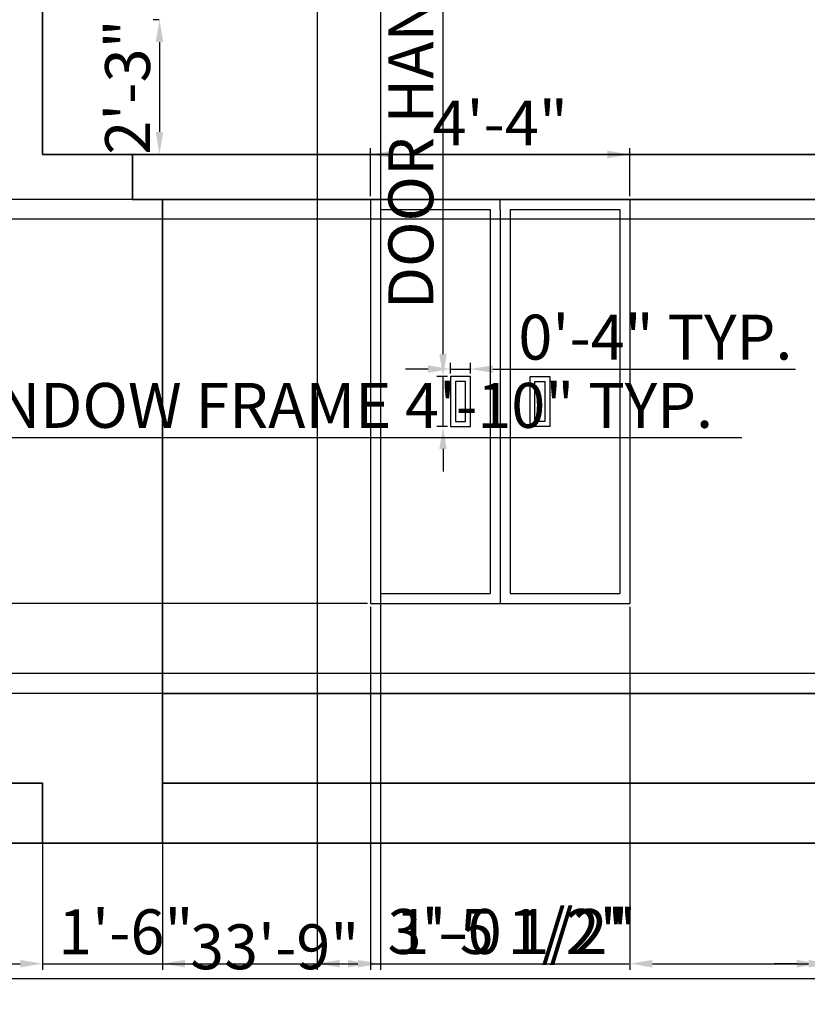
# Model space of a CAD drawing. Units: inches. Extents: x 3297 to 3846, y 520 to 959.
# Tile 2 of 5: x 3483 to 3641, y 520 to 717. Entities that reach past the tile are written whole.
import ezdxf

# ---------------------------------------------------------------- set-up
doc = ezdxf.new("R2010")
doc.units = ezdxf.units.IN
for name, color, linetype, lineweight in [('A-ANNO-DIMS', 2, 'Continuous', 18), ('A-DOOR', 4, 'Continuous', 25), ('A-ELEV', 7, 'Continuous', 35)]:
    doc.layers.add(name, color=color, linetype=linetype, lineweight=lineweight)
doc.styles.get("Standard").update_dxf_attribs({"font": 'arial.ttf'})
doc.dimstyles.new('ISO-25', dxfattribs={"dimtxt": 9, "dimasz": 4.5, "dimexe": 1.25, "dimexo": 0.625, "dimtad": 1, "dimdec": 0, "dimlunit": 3, "dimtxsty": 'Standard', "dimcen": 2.5, "dimadec": 0, "dimazin": 0, "dimtfac": 1, "dimtdec": 0, "dimtmove": 0, "dimatfit": 3, "dimfxl": 1, "dimarcsym": 0})

# ---------------------------------------------------------------- blocks, each defined once
blk = doc.blocks.new('*D7')
at = {"layer": 'A-ANNO-DIMS', "color": 0, "lineweight": -2, "transparency": 16777216}
for p, q in [((3332.06, 551.62), (3332.06, 523.84)), ((3737.06, 551.62), (3737.06, 523.84)), ((3336.56, 525.09), (3732.56, 525.09))]:
    blk.add_line(p, q, dxfattribs=at)
at = {"layer": 'A-ANNO-DIMS', "color": 0, "transparency": 16777216}
for points in [[(3336.56, 525.84), (3336.56, 524.34), (3332.06, 525.09)], [(3732.56, 525.84), (3732.56, 524.34), (3737.06, 525.09)]]:
    blk.add_solid(points, dxfattribs=at)
at = {"layer": 'Defpoints', "color": 0, "transparency": 16777216}
for p in [(3332.06, 552.24), (3737.06, 552.24), (3737.06, 525.09)]:
    blk.add_point(p, dxfattribs=at)
at = {"layer": 'A-ANNO-DIMS', "color": 0, "transparency": 16777216, "insert": (3534.56, 530.31), "char_height": 9, "attachment_point": 5}
blk.add_mtext('33\'-9"', dxfattribs=at)
blk = doc.blocks.new('*D12')
at = {"layer": 'A-ANNO-DIMS', "color": 0, "lineweight": -2, "transparency": 16777216}
for p, q in [((3553.76, 681.87), (3553.76, 691.49)), ((3605.76, 681.87), (3605.76, 691.49)), ((3558.26, 690.24), (3601.26, 690.24))]:
    blk.add_line(p, q, dxfattribs=at)
at = {"layer": 'A-ANNO-DIMS', "color": 0, "transparency": 16777216}
for points in [[(3558.26, 690.99), (3558.26, 689.49), (3553.76, 690.24)], [(3601.26, 690.99), (3601.26, 689.49), (3605.76, 690.24)]]:
    blk.add_solid(points, dxfattribs=at)
at = {"layer": 'Defpoints', "color": 0, "transparency": 16777216}
for p in [(3605.76, 690.24), (3553.76, 681.24), (3605.76, 681.24)]:
    blk.add_point(p, dxfattribs=at)
at = {"layer": 'A-ANNO-DIMS', "color": 0, "transparency": 16777216, "insert": (3579.76, 695.37), "char_height": 9, "attachment_point": 5}
blk.add_mtext('4\'-4"', dxfattribs=at)
blk = doc.blocks.new('*D19')
at = {"layer": 'A-ANNO-DIMS', "color": 0, "lineweight": -2, "transparency": 16777216}
for p, q in [((3511.44, 717.24), (3510.23, 717.24)), ((3511.48, 712.74), (3511.48, 694.74)), ((3511.44, 690.24), (3510.23, 690.24))]:
    blk.add_line(p, q, dxfattribs=at)
at = {"layer": 'A-ANNO-DIMS', "color": 0, "transparency": 16777216}
for points in [[(3510.73, 712.74), (3512.23, 712.74), (3511.48, 717.24)], [(3510.73, 694.74), (3512.23, 694.74), (3511.48, 690.24)]]:
    blk.add_solid(points, dxfattribs=at)
at = {"layer": 'Defpoints', "color": 0, "transparency": 16777216}
for p in [(3512.06, 717.24), (3511.48, 690.24), (3512.06, 690.24)]:
    blk.add_point(p, dxfattribs=at)
at = {"layer": 'A-ANNO-DIMS', "color": 0, "transparency": 16777216, "insert": (3506.25, 703.74), "char_height": 9, "attachment_point": 5, "rotation": 90}
blk.add_mtext('2\'-3"', dxfattribs=at)
blk = doc.blocks.new('DOOR-HANDLE')
for points in [[(3573.8, 645.74), (3569.8, 645.74), (3569.8, 640.74), (3569.8, 635.74), (3573.8, 635.74), (3573.8, 640.74)], [(3572.8, 644.74), (3570.8, 644.74), (3570.8, 640.74), (3570.8, 636.74), (3572.8, 636.74), (3572.8, 640.74)]]:
    blk.add_lwpolyline(points, close=True)
blk = doc.blocks.new('*D29')
at = {"layer": 'A-ANNO-DIMS', "color": 0, "lineweight": -2, "transparency": 16777216}
for p, q in [((3568.3, 650.24), (3568.3, 813.1)), ((3569.18, 645.74), (3567.05, 645.74)), ((3568.3, 635.74), (3568.3, 645.74)), ((3569.18, 635.74), (3567.05, 635.74)), ((3568.3, 631.24), (3568.3, 626.74))]:
    blk.add_line(p, q, dxfattribs=at)
at = {"layer": 'A-ANNO-DIMS', "color": 0, "transparency": 16777216}
for points in [[(3567.55, 650.24), (3569.05, 650.24), (3568.3, 645.74)], [(3567.55, 631.24), (3569.05, 631.24), (3568.3, 635.74)]]:
    blk.add_solid(points, dxfattribs=at)
at = {"layer": 'Defpoints', "color": 0, "transparency": 16777216}
for p in [(3568.3, 645.74), (3569.8, 645.74), (3569.8, 635.74)]:
    blk.add_point(p, dxfattribs=at)
at = {"layer": 'A-ANNO-DIMS', "color": 0, "transparency": 16777216, "insert": (3563.02, 733.92), "char_height": 9, "attachment_point": 5, "rotation": 90}
blk.add_mtext('DOOR HANDLE 0\'-10" TYP.', dxfattribs=at)
blk = doc.blocks.new('*D30')
at = {"layer": 'A-ANNO-DIMS', "color": 0, "lineweight": -2, "transparency": 16777216}
for p, q in [((3565.3, 647.24), (3560.8, 647.24)), ((3569.8, 646.37), (3569.8, 648.49)), ((3569.8, 647.24), (3573.8, 647.24)), ((3573.8, 646.37), (3573.8, 648.49)), ((3578.3, 647.24), (3638.91, 647.24))]:
    blk.add_line(p, q, dxfattribs=at)
at = {"layer": 'A-ANNO-DIMS', "color": 0, "transparency": 16777216}
for points in [[(3565.3, 647.99), (3565.3, 646.49), (3569.8, 647.24)], [(3578.3, 647.99), (3578.3, 646.49), (3573.8, 647.24)]]:
    blk.add_solid(points, dxfattribs=at)
at = {"layer": 'Defpoints', "color": 0, "transparency": 16777216}
for p in [(3573.8, 647.24), (3569.8, 645.74), (3573.8, 645.74)]:
    blk.add_point(p, dxfattribs=at)
at = {"layer": 'A-ANNO-DIMS', "color": 0, "transparency": 16777216, "insert": (3610.86, 652.46), "char_height": 9, "attachment_point": 5}
blk.add_mtext('0\'-4" TYP.', dxfattribs=at)
blk = doc.blocks.new('*D31')
at = {"layer": 'A-ANNO-DIMS', "color": 0, "lineweight": -2, "transparency": 16777216}
for p, q in [((3396.06, 641.58), (3396.06, 632.26)), ((3454.06, 641.58), (3454.06, 632.26)), ((3400.56, 633.51), (3449.56, 633.51)), ((3454.06, 633.51), (3628.19, 633.51))]:
    blk.add_line(p, q, dxfattribs=at)
at = {"layer": 'A-ANNO-DIMS', "color": 0, "transparency": 16777216}
for points in [[(3400.56, 634.26), (3400.56, 632.76), (3396.06, 633.51)], [(3449.56, 634.26), (3449.56, 632.76), (3454.06, 633.51)]]:
    blk.add_solid(points, dxfattribs=at)
at = {"layer": 'Defpoints', "color": 0, "transparency": 16777216}
for p in [(3396.06, 642.21), (3454.06, 642.21), (3454.06, 633.51)]:
    blk.add_point(p, dxfattribs=at)
at = {"layer": 'A-ANNO-DIMS', "color": 0, "transparency": 16777216, "insert": (3543.38, 638.79), "char_height": 9, "attachment_point": 5}
blk.add_mtext('WINDOW FRAME 4\'-10" TYP.', dxfattribs=at)
blk = doc.blocks.new('*D51')
at = {"layer": 'A-ANNO-DIMS', "color": 0, "lineweight": -2, "transparency": 16777216}
for p, q in [((3646.06, 575.62), (3646.06, 526.84)), ((3643.69, 563.62), (3643.69, 526.84)), ((3639.19, 528.09), (3634.69, 528.09)), ((3643.69, 528.09), (3646.06, 528.09)), ((3650.56, 528.09), (3701.21, 528.09))]:
    blk.add_line(p, q, dxfattribs=at)
at = {"layer": 'A-ANNO-DIMS', "color": 0, "transparency": 16777216}
for points in [[(3639.19, 528.84), (3639.19, 527.34), (3643.69, 528.09)], [(3650.56, 528.84), (3650.56, 527.34), (3646.06, 528.09)]]:
    blk.add_solid(points, dxfattribs=at)
at = {"layer": 'Defpoints', "color": 0, "transparency": 16777216}
for p in [(3646.06, 576.24), (3643.69, 564.24), (3646.06, 528.09)]:
    blk.add_point(p, dxfattribs=at)
at = {"layer": 'A-ANNO-DIMS', "color": 0, "transparency": 16777216, "insert": (3678.14, 533.37), "char_height": 9, "attachment_point": 5}
blk.add_mtext('0\'-2 1/2"', dxfattribs=at)
blk = doc.blocks.new('*D52')
at = {"layer": 'A-ANNO-DIMS', "color": 0, "lineweight": -2, "transparency": 16777216}
for p, q in [((3553.76, 599.62), (3553.76, 526.84)), ((3512.06, 581.62), (3512.06, 526.84)), ((3516.56, 528.09), (3549.26, 528.09)), ((3553.76, 528.09), (3604.4, 528.09))]:
    blk.add_line(p, q, dxfattribs=at)
at = {"layer": 'A-ANNO-DIMS', "color": 0, "transparency": 16777216}
for points in [[(3516.56, 528.84), (3516.56, 527.34), (3512.06, 528.09)], [(3549.26, 528.84), (3549.26, 527.34), (3553.76, 528.09)]]:
    blk.add_solid(points, dxfattribs=at)
at = {"layer": 'Defpoints', "color": 0, "transparency": 16777216}
for p in [(3553.76, 600.24), (3512.06, 582.24), (3553.76, 528.09)]:
    blk.add_point(p, dxfattribs=at)
at = {"layer": 'A-ANNO-DIMS', "color": 0, "transparency": 16777216, "insert": (3581.33, 533.37), "char_height": 9, "attachment_point": 5}
blk.add_mtext('3\'-5 1/2"', dxfattribs=at)
blk = doc.blocks.new('*D53')
at = {"layer": 'A-ANNO-DIMS', "color": 0, "lineweight": -2, "transparency": 16777216}
for p, q in [((3605.76, 599.62), (3605.76, 526.84)), ((3646.06, 581.62), (3646.06, 526.84)), ((3610.26, 528.09), (3641.56, 528.09)), ((3646.06, 528.09), (3696.7, 528.09))]:
    blk.add_line(p, q, dxfattribs=at)
at = {"layer": 'A-ANNO-DIMS', "color": 0, "transparency": 16777216}
for points in [[(3610.26, 528.84), (3610.26, 527.34), (3605.76, 528.09)], [(3641.56, 528.84), (3641.56, 527.34), (3646.06, 528.09)]]:
    blk.add_solid(points, dxfattribs=at)
at = {"layer": 'Defpoints', "color": 0, "transparency": 16777216}
for p in [(3605.76, 600.24), (3646.06, 582.24), (3646.06, 528.09)]:
    blk.add_point(p, dxfattribs=at)
at = {"layer": 'A-ANNO-DIMS', "color": 0, "transparency": 16777216, "insert": (3673.63, 533.37), "char_height": 9, "attachment_point": 5}
blk.add_mtext('3\'-4 1/2"', dxfattribs=at)
blk = doc.blocks.new('*D55')
at = {"layer": 'A-ANNO-DIMS', "color": 0, "lineweight": -2, "transparency": 16777216}
for p, q in [((3553.14, 681.24), (3306.66, 681.24)), ((3307.91, 604.74), (3307.91, 676.74)), ((3553.14, 600.24), (3306.66, 600.24))]:
    blk.add_line(p, q, dxfattribs=at)
at = {"layer": 'A-ANNO-DIMS', "color": 0, "transparency": 16777216}
for points in [[(3307.16, 676.74), (3308.66, 676.74), (3307.91, 681.24)], [(3307.16, 604.74), (3308.66, 604.74), (3307.91, 600.24)]]:
    blk.add_solid(points, dxfattribs=at)
at = {"layer": 'Defpoints', "color": 0, "transparency": 16777216}
for p in [(3307.91, 681.24), (3553.76, 681.24), (3553.76, 600.24)]:
    blk.add_point(p, dxfattribs=at)
at = {"layer": 'A-ANNO-DIMS', "color": 0, "transparency": 16777216, "insert": (3302.69, 640.74), "char_height": 9, "attachment_point": 5, "rotation": 90}
blk.add_mtext('6\'-9"', dxfattribs=at)
blk = doc.blocks.new('*D56')
at = {"layer": 'A-ANNO-DIMS', "color": 0, "lineweight": -2, "transparency": 16777216}
for p, q in [((3307.91, 600.24), (3307.91, 629.07)), ((3553.14, 600.24), (3306.66, 600.24)), ((3307.91, 586.74), (3307.91, 595.74)), ((3511.44, 582.24), (3306.66, 582.24))]:
    blk.add_line(p, q, dxfattribs=at)
at = {"layer": 'A-ANNO-DIMS', "color": 0, "transparency": 16777216}
for points in [[(3307.16, 595.74), (3308.66, 595.74), (3307.91, 600.24)], [(3307.16, 586.74), (3308.66, 586.74), (3307.91, 582.24)]]:
    blk.add_solid(points, dxfattribs=at)
at = {"layer": 'Defpoints', "color": 0, "transparency": 16777216}
for p in [(3307.91, 600.24), (3553.76, 600.24), (3512.06, 582.24)]:
    blk.add_point(p, dxfattribs=at)
at = {"layer": 'A-ANNO-DIMS', "color": 0, "transparency": 16777216, "insert": (3302.69, 616.9), "char_height": 9, "attachment_point": 5, "rotation": 90}
blk.add_mtext('1\'-6"', dxfattribs=at)
blk = doc.blocks.new('*D57')
at = {"layer": 'A-ANNO-DIMS', "color": 0, "lineweight": -2, "transparency": 16777216}
for p, q in [((3645.44, 681.24), (3306.66, 681.24)), ((3307.91, 586.74), (3307.91, 676.74)), ((3645.44, 582.24), (3306.66, 582.24))]:
    blk.add_line(p, q, dxfattribs=at)
at = {"layer": 'A-ANNO-DIMS', "color": 0, "transparency": 16777216}
for points in [[(3307.16, 676.74), (3308.66, 676.74), (3307.91, 681.24)], [(3307.16, 586.74), (3308.66, 586.74), (3307.91, 582.24)]]:
    blk.add_solid(points, dxfattribs=at)
at = {"layer": 'Defpoints', "color": 0, "transparency": 16777216}
for p in [(3307.91, 681.24), (3646.06, 681.24), (3646.06, 582.24)]:
    blk.add_point(p, dxfattribs=at)
at = {"layer": 'A-ANNO-DIMS', "color": 0, "transparency": 16777216, "insert": (3302.69, 631.74), "char_height": 9, "attachment_point": 5, "rotation": 90}
blk.add_mtext('8\'-3"', dxfattribs=at)
blk = doc.blocks.new('*D59')
at = {"layer": 'A-ANNO-DIMS', "color": 0, "lineweight": -2, "transparency": 16777216}
for p, q in [((3649.439671, 677.241209), (3306.664671, 677.241209)), ((3307.914671, 590.741209), (3307.914671, 672.741209)), ((3649.439671, 586.241209), (3306.664671, 586.241209))]:
    blk.add_line(p, q, dxfattribs=at)
at = {"layer": 'A-ANNO-DIMS', "color": 0, "transparency": 16777216}
for points in [[(3307.164671, 672.741209), (3308.664671, 672.741209), (3307.914671, 677.241209)], [(3307.164671, 590.741209), (3308.664671, 590.741209), (3307.914671, 586.241209)]]:
    blk.add_solid(points, dxfattribs=at)
at = {"layer": 'Defpoints', "color": 0, "transparency": 16777216}
for p in [(3307.914671, 677.241209), (3650.064671, 677.241209), (3650.064671, 586.241209)]:
    blk.add_point(p, dxfattribs=at)
at = {"layer": 'A-ANNO-DIMS', "color": 0, "transparency": 16777216, "insert": (3302.789671, 631.741209), "char_height": 9, "attachment_point": 5, "rotation": 90}
blk.add_mtext('7\'-7"', dxfattribs=at)
blk = doc.blocks.new('*D70')
at = {"layer": 'A-ANNO-DIMS', "color": 0, "lineweight": -2, "transparency": 16777216}
for p, q in [((3555.76, 760.62), (3555.76, 526.84)), ((3543.06, 758.62), (3543.06, 526.84)), ((3547.56, 528.09), (3551.26, 528.09)), ((3555.76, 528.09), (3605.56, 528.09))]:
    blk.add_line(p, q, dxfattribs=at)
at = {"layer": 'A-ANNO-DIMS', "color": 0, "transparency": 16777216}
for points in [[(3547.56, 528.84), (3547.56, 527.34), (3543.06, 528.09)], [(3551.26, 528.84), (3551.26, 527.34), (3555.76, 528.09)]]:
    blk.add_solid(points, dxfattribs=at)
at = {"layer": 'Defpoints', "color": 0, "transparency": 16777216}
for p in [(3555.76, 761.24), (3543.06, 759.24), (3555.76, 528.09)]:
    blk.add_point(p, dxfattribs=at)
at = {"layer": 'A-ANNO-DIMS', "color": 0, "transparency": 16777216, "insert": (3582.91, 533.37), "char_height": 9, "attachment_point": 5}
blk.add_mtext('1\'-0 1/2"', dxfattribs=at)
blk = doc.blocks.new('*D77')
at = {"layer": 'A-ANNO-DIMS', "color": 0, "lineweight": -2, "transparency": 16777216}
for p, q in [((3470.06, 563.62), (3470.06, 526.84)), ((3488.06, 563.62), (3488.06, 526.84)), ((3474.56, 528.09), (3483.56, 528.09)), ((3488.06, 528.09), (3516.89, 528.09))]:
    blk.add_line(p, q, dxfattribs=at)
at = {"layer": 'A-ANNO-DIMS', "color": 0, "transparency": 16777216}
for points in [[(3474.56, 528.84), (3474.56, 527.34), (3470.06, 528.09)], [(3483.56, 528.84), (3483.56, 527.34), (3488.06, 528.09)]]:
    blk.add_solid(points, dxfattribs=at)
at = {"layer": 'Defpoints', "color": 0, "transparency": 16777216}
for p in [(3470.06, 564.24), (3488.06, 564.24), (3488.06, 528.09)]:
    blk.add_point(p, dxfattribs=at)
at = {"layer": 'A-ANNO-DIMS', "color": 0, "transparency": 16777216, "insert": (3504.73, 533.31), "char_height": 9, "attachment_point": 5}
blk.add_mtext('1\'-6"', dxfattribs=at)
blk = doc.blocks.new('*D79')
at = {"layer": 'A-ANNO-DIMS', "color": 0, "lineweight": -2, "transparency": 16777216}
for p, q in [((3307.91, 564.24), (3307.91, 593.07)), ((3487.44, 564.24), (3306.66, 564.24)), ((3307.91, 556.74), (3307.91, 559.74)), ((3487.44, 552.24), (3306.66, 552.24))]:
    blk.add_line(p, q, dxfattribs=at)
at = {"layer": 'A-ANNO-DIMS', "color": 0, "transparency": 16777216}
for points in [[(3307.16, 559.74), (3308.66, 559.74), (3307.91, 564.24)], [(3307.16, 556.74), (3308.66, 556.74), (3307.91, 552.24)]]:
    blk.add_solid(points, dxfattribs=at)
at = {"layer": 'Defpoints', "color": 0, "transparency": 16777216}
for p in [(3307.91, 564.24), (3488.06, 564.24), (3488.06, 552.24)]:
    blk.add_point(p, dxfattribs=at)
at = {"layer": 'A-ANNO-DIMS', "color": 0, "transparency": 16777216, "insert": (3302.69, 580.9), "char_height": 9, "attachment_point": 5, "rotation": 90}
blk.add_mtext('1\'-0"', dxfattribs=at)

msp = doc.modelspace()

# ---------------------------------------------------------------- linework, layer by layer
at = {"layer": 'A-DOOR'}
for p, q in [((3553.76, 681.24), (3553.76, 600.24)), ((3579.76, 679.24), (3579.76, 681.24)), ((3605.76, 681.24), (3605.76, 600.24)), ((3555.76, 679.24), (3555.76, 602.24)), ((3555.76, 679.24), (3577.76, 679.24)), ((3555.76, 679.24), (3577.76, 679.24)), ((3577.76, 679.24), (3577.76, 602.24)), ((3579.76, 679.24), (3579.76, 600.24)), ((3581.76, 679.24), (3581.76, 602.24)), ((3581.76, 679.24), (3603.76, 679.24)), ((3603.76, 679.24), (3603.76, 602.24)), ((3555.76, 602.24), (3577.76, 602.24)), ((3581.76, 602.24), (3603.76, 602.24)), ((3553.76, 600.24), (3605.76, 600.24))]:
    msp.add_line(p, q, dxfattribs=at)
at = {"layer": 'A-ELEV'}
for p, q in [((3488.06, 690.24), (3488.06, 872.24)), ((3488.06, 690.24), (3752.06, 690.24)), ((3506.06, 690.24), (3506.06, 681.24)), ((3506.06, 681.24), (3752.06, 681.24)), ((3512.06, 681.24), (3512.06, 552.24)), ((3512.06, 582.24), (3718.06, 582.24)), ((3332.06, 564.24), (3488.06, 564.24)), ((3488.06, 564.24), (3488.06, 552.24)), ((3512.06, 564.24), (3737.06, 564.24)), ((3332.06, 552.24), (3737.06, 552.24))]:
    msp.add_line(p, q, dxfattribs=at)

# ---------------------------------------------------------------- block references
at = {"layer": 'A-DOOR'}
msp.add_blockref('DOOR-HANDLE', (0, 0), dxfattribs=at)
at = {"layer": 'A-DOOR', "extrusion": (0, 0, -1), "zscale": -1}
msp.add_blockref('DOOR-HANDLE', (-7159.53, 0), dxfattribs=at)

# ---------------------------------------------------------------- dimensions: what is measured, and where the dimension line sits
at = {"layer": 'A-ANNO-DIMS'}
dim = msp.add_linear_dim(base=(3568.3, 645.74), p1=(3569.8, 635.74), p2=(3569.8, 645.74), angle=90, text='DOOR HANDLE <> TYP.', dimstyle='ISO-25', override={"dimdec": 1, "dimrnd": 0, "dimzin": 1, "dimlunit": 4, "dimfrac": 2}, dxfattribs=at)
dim.commit()
dim.dimension.update_dxf_attribs({"geometry": '*D29', "text_midpoint": (3563.02, 733.92)})
for base, p1, p2, override, picture, middle in [((3555.76, 528.09), (3543.06, 759.24), (3555.76, 761.24), {"dimdec": 1, "dimlfac": 1, "dimrnd": 0, "dimzin": 1, "dimdsep": 46, "dimlunit": 4, "dimfrac": 2}, '*D70', (3582.91, 533.37)), ((3605.76, 690.24), (3553.76, 681.24), (3605.76, 681.24), {"dimclrd": 0, "dimclre": 0, "dimclrt": 0}, '*D12', (3579.76, 695.37)), ((3553.76, 528.09), (3512.06, 582.24), (3553.76, 600.24), {"dimdec": 1, "dimlfac": 1, "dimrnd": 0, "dimzin": 1, "dimdsep": 46, "dimlunit": 4, "dimfrac": 2}, '*D52', (3581.33, 533.37)), ((3646.06, 528.09), (3605.76, 600.24), (3646.06, 582.24), {"dimdec": 1, "dimlfac": 1, "dimrnd": 0, "dimzin": 1, "dimdsep": 46, "dimlunit": 4, "dimfrac": 2}, '*D53', (3673.63, 533.37)), ((3646.06, 528.09), (3643.69, 564.24), (3646.06, 576.24), {"dimdec": 1, "dimlfac": 1, "dimrnd": 0, "dimzin": 1, "dimdsep": 46, "dimlunit": 4, "dimfrac": 2}, '*D51', (3678.14, 533.37)), ((3488.06, 528.09), (3470.06, 564.24), (3488.06, 564.24), {"dimdec": 1, "dimlfac": 1, "dimrnd": 0, "dimzin": 1, "dimdsep": 46, "dimlunit": 4, "dimfrac": 2}, '*D77', (3504.73, 533.31)), ((3737.06, 525.09), (3332.06, 552.24), (3737.06, 552.24), {"dimclrd": 0, "dimclre": 0, "dimclrt": 0}, '*D7', (3534.56, 530.31))]:
    dim = msp.add_linear_dim(base=base, p1=p1, p2=p2, dimstyle='ISO-25', override=override, dxfattribs=at)
    dim.commit()
    dim.dimension.update_dxf_attribs({"geometry": picture, "text_midpoint": middle})
for base, p1, p2, override, picture, middle in [((3511.48, 690.24), (3512.06, 717.24), (3512.06, 690.24), {"dimclrd": 0, "dimclre": 0, "dimclrt": 0}, '*D19', (3506.25, 703.74)), ((3307.91, 681.24), (3553.76, 600.24), (3553.76, 681.24), {"dimdec": 1, "dimlfac": 1, "dimrnd": 0, "dimzin": 1, "dimdsep": 46, "dimlunit": 4, "dimfrac": 2}, '*D55', (3302.69, 640.74)), ((3307.91, 681.24), (3646.06, 582.24), (3646.06, 681.24), {"dimdec": 1, "dimlfac": 1, "dimrnd": 0, "dimzin": 1, "dimdsep": 46, "dimlunit": 4, "dimfrac": 2}, '*D57', (3302.69, 631.74)), ((3307.91, 677.24), (3650.06, 586.24), (3650.06, 677.24), {"dimdec": 1, "dimlfac": 1, "dimrnd": 0, "dimzin": 1, "dimdsep": 46, "dimlunit": 4, "dimfrac": 2}, '*D59', (3302.79, 631.74)), ((3307.91, 600.24), (3512.06, 582.24), (3553.76, 600.24), {"dimdec": 1, "dimlfac": 1, "dimrnd": 0, "dimzin": 1, "dimdsep": 46, "dimlunit": 4, "dimfrac": 2}, '*D56', (3302.69, 616.9)), ((3307.91, 564.24), (3488.06, 552.24), (3488.06, 564.24), {"dimdec": 1, "dimlfac": 1, "dimrnd": 0, "dimzin": 1, "dimdsep": 46, "dimlunit": 4, "dimfrac": 2}, '*D79', (3302.69, 580.9))]:
    dim = msp.add_linear_dim(base=base, p1=p1, p2=p2, angle=90, dimstyle='ISO-25', override=override, dxfattribs=at)
    dim.commit()
    dim.dimension.update_dxf_attribs({"geometry": picture, "text_midpoint": middle})
for base, p1, p2, text, picture, middle in [((3454.06, 633.51), (3396.06, 642.21), (3454.06, 642.21), 'WINDOW FRAME <> TYP.', '*D31', (3543.38, 638.79)), ((3573.8, 647.24), (3569.8, 645.74), (3573.8, 645.74), '<> TYP.', '*D30', (3610.86, 652.46))]:
    dim = msp.add_linear_dim(base=base, p1=p1, p2=p2, text=text, dimstyle='ISO-25', override={"dimdec": 1, "dimrnd": 0, "dimzin": 1, "dimlunit": 4, "dimfrac": 2}, dxfattribs=at)
    dim.commit()
    dim.dimension.update_dxf_attribs({"geometry": picture, "text_midpoint": middle})

doc.saveas('drawing.dxf')
